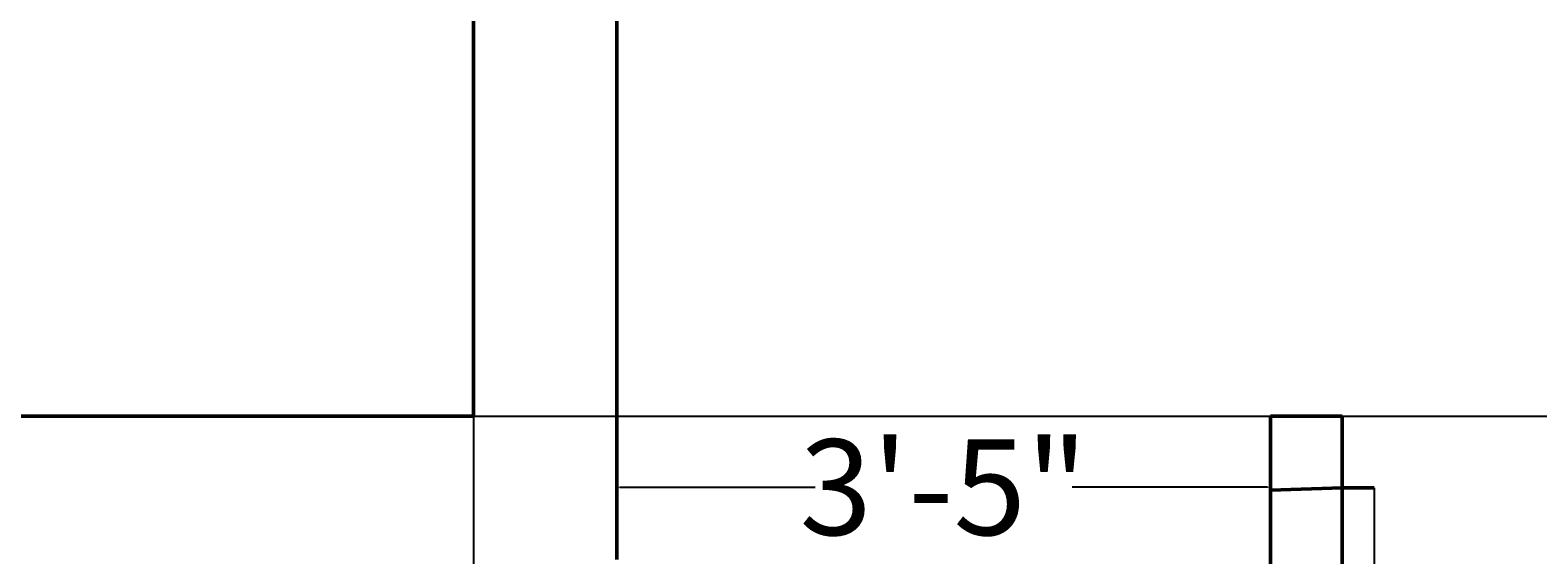
# Model space of a CAD drawing. Units: inches. Extents: x -173 to 545, y -746 to 104.
# Tile 15 of 32: x 278 to 373, y -561 to -528. Entities that reach past the tile are written whole.
import ezdxf

# ---------------------------------------------------------------- set-up
doc = ezdxf.new("R2010")
doc.units = ezdxf.units.IN
doc.header["$MEASUREMENT"] = 0
for name, color, linetype, lineweight in [('A-ANNO-DIMS', 2, 'Continuous', 18), ('A-DOOR', 4, 'Continuous', 25), ('A-WALL', 7, 'Continuous', 50)]:
    doc.layers.add(name, color=color, linetype=linetype, lineweight=lineweight)
doc.styles.get("Standard").update_dxf_attribs({"font": 'arial.ttf'})
doc.dimstyles.get("Standard").update_dxf_attribs({"dimtxt": 0.18, "dimasz": 0.18, "dimexe": 0.18, "dimexo": 0.0625, "dimgap": 0.09, "dimtad": 0, "dimtih": 1, "dimtoh": 1, "dimdec": 0, "dimzin": 0, "dimdsep": 46, "dimlunit": 3, "dimtxsty": 'Standard', "dimcen": 0.09, "dimadec": 0, "dimazin": 0, "dimtfac": 1, "dimtdec": 0, "dimtofl": 0, "dimtmove": 0, "dimatfit": 3, "dimfxl": 1, "dimtolj": 1, "dimtzin": 0, "dimarcsym": 0})

# ---------------------------------------------------------------- blocks, each defined once
blk = doc.blocks.new('*D16')
at = {"layer": 'A-ANNO-DIMS', "color": 0, "lineweight": -2, "transparency": 16777216}
for p, q in [((315.301, -551.924), (315.301, -556.504)), ((356.301, -551.924), (356.301, -556.504)), ((315.481, -556.324), (327.739, -556.324)), ((356.121, -556.324), (343.864, -556.324))]:
    blk.add_line(p, q, dxfattribs=at)
at = {"layer": 'A-ANNO-DIMS', "color": 0, "transparency": 16777216}
for points in [[(315.481, -556.294), (315.481, -556.354), (315.301, -556.324)], [(356.121, -556.294), (356.121, -556.354), (356.301, -556.324)]]:
    blk.add_solid(points, dxfattribs=at)
at = {"layer": 'Defpoints', "color": 0, "transparency": 16777216}
for p in [(315.301, -551.862), (356.301, -551.862), (356.301, -556.324)]:
    blk.add_point(p, dxfattribs=at)
at = {"layer": 'A-ANNO-DIMS', "color": 0, "transparency": 16777216, "insert": (335.801, -556.324), "char_height": 6, "attachment_point": 5}
blk.add_mtext('\\A1;3\'-5"', dxfattribs=at)
blk = doc.blocks.new('DOOR-24')
blk.add_line((24, 0), (24, 24))
blk.add_arc((24, 0), 24, 90, 180)
blk = doc.blocks.new('*D81')
at = {"layer": 'A-ANNO-DIMS', "color": 0, "lineweight": -2, "transparency": 16777216}
for p, q in [((219.801, -551.924), (219.801, -740.642)), ((306.301, -551.924), (306.301, -740.642)), ((219.981, -740.462), (262.513, -740.462)), ((306.121, -740.462), (263.59, -740.462))]:
    blk.add_line(p, q, dxfattribs=at)
at = {"layer": 'A-ANNO-DIMS', "color": 0, "transparency": 16777216}
for points in [[(219.981, -740.432), (219.981, -740.492), (219.801, -740.462)], [(306.121, -740.432), (306.121, -740.492), (306.301, -740.462)]]:
    blk.add_solid(points, dxfattribs=at)
at = {"layer": 'Defpoints', "color": 0, "transparency": 16777216}
for p in [(219.801, -551.862), (306.301, -551.862), (306.301, -740.462)]:
    blk.add_point(p, dxfattribs=at)
at = {"layer": 'A-ANNO-DIMS', "color": 0, "transparency": 16777216, "insert": (263.051, -740.462), "char_height": 0.18, "attachment_point": 5}
blk.add_mtext('\\A1;7\'-2 1/2"', dxfattribs=at)
blk = doc.blocks.new('*D82')
at = {"layer": 'A-ANNO-DIMS', "color": 0, "lineweight": -2, "transparency": 16777216}
for p, q in [((219.864, -467.862), (545.081, -467.862)), ((544.901, -468.042), (544.901, -509.68)), ((544.901, -551.682), (544.901, -510.044)), ((219.864, -551.862), (545.081, -551.862))]:
    blk.add_line(p, q, dxfattribs=at)
at = {"layer": 'A-ANNO-DIMS', "color": 0, "transparency": 16777216}
for points in [[(544.871, -468.042), (544.931, -468.042), (544.901, -467.862)], [(544.871, -551.682), (544.931, -551.682), (544.901, -551.862)]]:
    blk.add_solid(points, dxfattribs=at)
at = {"layer": 'Defpoints', "color": 0, "transparency": 16777216}
for p in [(219.801, -467.862), (219.801, -551.862), (544.901, -551.862)]:
    blk.add_point(p, dxfattribs=at)
at = {"layer": 'A-ANNO-DIMS', "color": 0, "transparency": 16777216, "insert": (544.901, -509.862), "char_height": 0.18, "attachment_point": 5}
blk.add_mtext('\\A1;7\'-0"', dxfattribs=at)

msp = doc.modelspace()

# ---------------------------------------------------------------- linework, layer by layer
at = {"layer": 'A-WALL'}
for p, q in [((315.301, -463.362), (315.301, -560.862)), ((306.301, -467.862), (306.301, -551.862)), ((219.801, -551.862), (306.301, -551.862)), ((356.301, -551.862), (356.301, -688.362)), ((360.801, -551.862), (356.301, -551.862)), ((360.801, -551.862), (360.801, -688.362)), ((360.801, -556.362), (356.301, -556.504)), ((360.801, -556.362), (362.801, -556.362))]:
    msp.add_line(p, q, dxfattribs=at)

# ---------------------------------------------------------------- block references
at = {"layer": 'A-DOOR', "rotation": 180}
msp.add_blockref('DOOR-24', (386.802, -556.362), dxfattribs=at)

# ---------------------------------------------------------------- dimensions: what is measured, and where the dimension line sits
at = {"layer": 'A-ANNO-DIMS'}
dim = msp.add_linear_dim(base=(544.901, -551.862), p1=(219.801, -467.862), p2=(219.801, -551.862), angle=90, dimstyle='Standard', override={"dimdec": 1, "dimlfac": 1, "dimrnd": 0, "dimzin": 1, "dimdsep": 46, "dimlunit": 4, "dimfrac": 2}, dxfattribs=at)
dim.commit()
dim.dimension.update_dxf_attribs({"geometry": '*D82', "text_midpoint": (544.901, -509.862)})
for base, p1, p2, override, picture, middle in [((306.301, -740.462), (219.801, -551.862), (306.301, -551.862), {"dimdec": 1, "dimlfac": 1, "dimrnd": 0, "dimzin": 1, "dimdsep": 46, "dimlunit": 4, "dimfrac": 2}, '*D81', (263.051, -740.462)), ((356.301, -556.324), (315.301, -551.862), (356.301, -551.862), {"dimtxt": 6, "dimclrd": 0, "dimclre": 0, "dimclrt": 0}, '*D16', (335.801, -556.324))]:
    dim = msp.add_linear_dim(base=base, p1=p1, p2=p2, dimstyle='Standard', override=override, dxfattribs=at)
    dim.commit()
    dim.dimension.update_dxf_attribs({"geometry": picture, "text_midpoint": middle})

doc.saveas('drawing.dxf')
